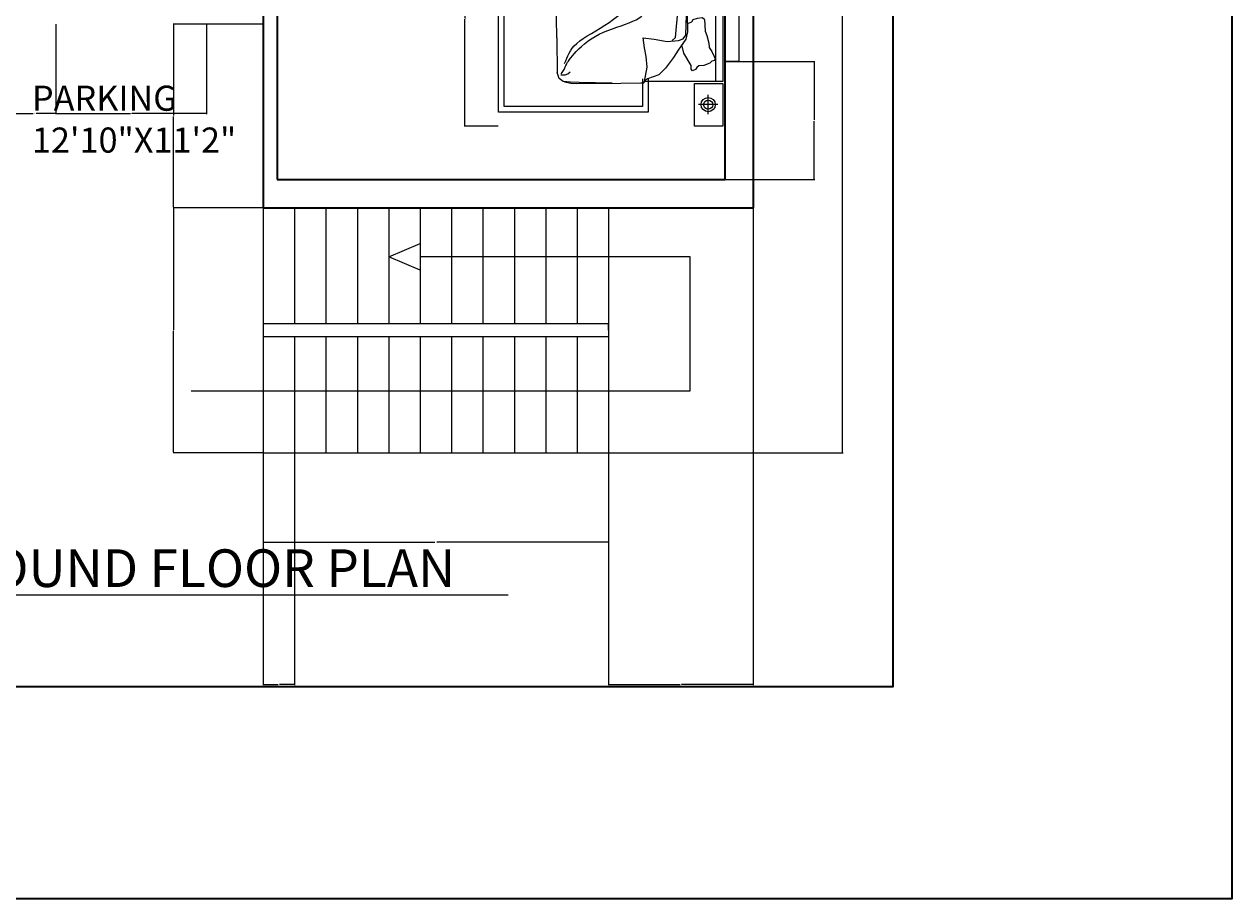
# Model space of a CAD drawing. Units: inches. Extents: x 1976 to 2558, y -977 to 2909.
# Tile 3 of 8: x 2173 to 2558, y 1748 to 2026. Entities that reach past the tile are written whole.
import ezdxf

# ---------------------------------------------------------------- set-up
doc = ezdxf.new("R2010")
doc.units = ezdxf.units.IN
for name, color, linetype, lineweight in [('A-ANNO-DIMS', 2, 'Continuous', 18), ('A-ANNO-SYMB', 2, 'Continuous', 18), ('A-ANNO-TEXT', 7, 'Continuous', 25), ('A-ANNO-TTLB', 7, 'Continuous', 35), ('A-AREA-IDEN', 7, 'Continuous', 18), ('A-FLOR-STRS', 7, 'Continuous', 25), ('A-FURN', 8, 'Continuous', 13), ('A-GLAZ', 4, 'Continuous', 18), ('A-WALL', 7, 'Continuous', 35)]:
    doc.layers.add(name, color=color, linetype=linetype, lineweight=lineweight)
doc.styles.get("Standard").update_dxf_attribs({"font": 'arial.ttf'})
doc.dimstyles.get("Standard").update_dxf_attribs({"dimtxt": 0.18, "dimasz": 0.18, "dimexe": 0.18, "dimexo": 0.0625, "dimgap": 0.09, "dimtad": 0, "dimtih": 1, "dimtoh": 1, "dimdec": 4, "dimzin": 0, "dimdsep": 46, "dimtxsty": 'Standard', "dimcen": 0.09, "dimadec": 0, "dimazin": 0, "dimtfac": 1, "dimtdec": 4, "dimtofl": 0, "dimtmove": 0, "dimatfit": 3, "dimfxl": 1, "dimtolj": 1, "dimtzin": 0, "dimarcsym": 0})

# ---------------------------------------------------------------- blocks, each defined once
blk = doc.blocks.new('BED-DOUBLE')
for p, q in [((69.87, 61.62), (63.73, 61.62)), ((66.8, 64.69), (66.8, 58.55)), ((20.15, 54.74), (18.94, 53.75)), ((22.42, 54.99), (20.15, 54.74)), ((25.18, 55.14), (22.42, 54.99)), ((35.73, 55.56), (25.18, 55.14)), ((55.41, 55.48), (35.73, 55.56)), ((56.88, 55.5), (55.41, 55.48)), ((57.51, 55.44), (56.88, 55.5)), ((58.41, 54.87), (71.47, 54.87)), ((18.94, 53.75), (18.3, 51.82)), ((18.55, 28.1), (18.3, 51.82)), ((66.5, 51.13), (67.81, 51.48)), ((60.75, 39.09), (59.91, 42.39)), ((68.04, 39.26), (68.74, 42.58)), ((68.74, 42.58), (68.6, 43.82)), ((60.42, 38.05), (60.75, 39.09)), ((68.42, 38.23), (68.04, 39.26)), ((60.63, 37.41), (60.42, 38.05)), ((61.72, 37.48), (60.63, 37.41)), ((62.3, 37.93), (61.72, 37.48)), ((63.04, 38.19), (62.3, 37.93)), ((64.58, 37.82), (63.04, 38.19)), ((66.65, 37.8), (64.58, 37.82)), ((67.64, 38.21), (66.65, 37.8)), ((68.39, 38.13), (67.64, 38.21)), ((68.39, 38.13), (67.64, 38.21)), ((68.39, 38.13), (68.42, 38.23)), ((65.64, 33.99), (65.86, 30.18)), ((18.55, 28.1), (18.55, 23.26)), ((65.86, 30.18), (66.35, 28.89)), ((66.35, 28.89), (67.01, 26.44)), ((18.55, 23.26), (18.68, 21.54)), ((61.33, 19.24), (59.08, 23.24)), ((67.01, 26.44), (67.13, 25.01)), ((67.13, 25.01), (67.97, 23.75)), ((67.13, 25.01), (67.97, 23.75)), ((67.97, 23.75), (68.81, 21.95)), ((18.68, 21.54), (18.68, 17.02)), ((61.37, 18.14), (61.33, 19.24)), ((65.36, 19.33), (63.79, 19.16)), ((67.32, 20.02), (65.36, 19.33)), ((68.1, 20.74), (67.32, 20.02)), ((19.39, 15.11), (18.68, 17.02)), ((19.85, 16.29), (21.2, 16.35)), ((21.2, 16.35), (22.12, 16.65)), ((22.12, 16.65), (22.82, 17.31)), ((61.78, 17.61), (61.37, 18.14)), ((62.78, 18.04), (61.78, 17.61)), ((63.18, 18.67), (62.78, 18.04)), ((63.79, 19.16), (63.18, 18.67)), ((20.62, 14.15), (19.39, 15.11)), ((22.9, 13.97), (20.62, 14.15)), ((21.04, 14.04), (23.05, 13.66)), ((25.67, 13.91), (22.9, 13.97)), ((23.05, 13.66), (24.99, 13.54)), ((24.99, 13.54), (38.97, 13.68)), ((36.23, 13.64), (25.67, 13.91)), ((38.97, 13.68), (45.35, 13.75)), ((46.53, 14.29), (46.57, 14.2)), ((66.8, 3.77), (66.8, 9.91)), ((69.87, 6.84), (63.73, 6.84))]:
    blk.add_line(p, q)
for points in [[(62.44, 68.46), (62.44, 54.92), (71.47, 54.92), (71.47, 68.46)], [(62.44, 0), (62.44, 13.54), (71.47, 13.54), (71.47, 0)]]:
    blk.add_lwpolyline(points, close=True)
for points in [[(47.73, 15.09), (47.73, 4.46), (0, 4.46), (0, 62.42), (47.73, 62.42), (47.73, 55.51)], [(45.92, 15.09), (45.92, 6.27), (1.81, 6.27), (1.81, 60.61), (45.92, 60.61), (45.92, 55.51)], [(46.51, 14.22), (47.31, 18.77), (47.06, 22.14), (46.5, 24.88), (46.05, 28.14), (49.6, 27.7), (53.74, 26.97), (57.39, 27.29), (58.87, 27.77), (59.72, 28.96), (59.98, 38.59), (59.57, 52.44), (58.73, 53.86), (57.9, 54.46), (57.82, 54.53)], [(58.65, 54.52), (59.13, 53.97), (59.77, 52.45), (60.21, 29.99), (59.63, 27.73), (57.24, 24.13), (55.74, 21.86), (53.24, 18.45), (51.03, 16.28), (47.47, 15), (46.54, 14.37)], [(71.47, 54.87), (71.47, 14.22), (46.61, 14.22)], [(55.37, 27.24), (56.41, 28.26), (57.19, 37.43), (57.04, 40.1), (56.37, 53.37), (55.53, 54.49), (54.4, 55.34)], [(57.55, 55.42), (57.97, 55.29), (58.3, 55.1), (58.41, 54.87), (58.64, 54.6), (58.65, 54.56)], [(69.21, 14.22), (69.21, 54.87)], [(59.99, 43.62), (60.51, 48.57), (60.69, 50), (60.38, 50.84), (60.47, 51.53), (61.01, 51.34), (61.95, 51.45), (64.12, 51.49), (66.5, 51.18)], [(68.6, 43.82), (67.86, 48.73), (67.62, 50.16), (67.9, 51.01), (67.81, 51.48)], [(21.07, 19.9), (21.44, 20.76), (21.79, 21.6), (22.14, 22.42), (22.52, 23.22), (22.95, 24.01), (23.48, 24.78), (24.13, 25.56), (24.93, 26.33), (25.9, 27.1), (27.01, 27.89), (28.25, 28.69), (29.59, 29.5), (30.98, 30.34), (32.41, 31.2), (33.84, 32.1), (35.25, 33.03), (36.61, 34), (37.91, 35), (39.14, 36), (40.28, 37), (41.34, 37.97), (42.3, 38.91), (43.16, 39.79), (43.9, 40.61), (44.52, 41.34), (44.99, 41.98), (45.3, 42.54), (45.43, 43.02), (45.35, 43.42), (45.05, 43.74), (44.51, 43.98), (43.7, 44.14)], [(20, 16.69), (20.29, 17.07), (20.52, 17.41), (20.72, 17.72), (20.88, 18.01), (21.02, 18.28), (21.14, 18.55), (21.26, 18.81), (21.37, 19.07), (21.5, 19.34), (21.64, 19.63), (21.82, 19.96), (22.04, 20.32), (22.31, 20.72), (22.64, 21.19), (23.05, 21.72), (23.54, 22.32), (24.12, 23.01), (24.8, 23.76), (25.57, 24.56), (26.43, 25.38), (27.39, 26.22), (28.43, 27.04), (29.56, 27.83), (30.78, 28.58), (32.09, 29.26), (33.45, 29.88), (34.86, 30.45), (36.28, 30.99), (37.7, 31.49), (39.08, 31.98), (40.41, 32.45), (41.66, 32.92), (42.81, 33.4), (43.84, 33.89), (44.73, 34.4), (45.46, 34.92), (46.02, 35.46), (46.39, 36.02), (46.55, 36.61), (46.48, 37.23)], [(65.64, 33.99), (64.89, 34.52), (63.32, 34.27), (61.94, 33.89), (61.5, 33.14), (60.37, 32.7), (60.16, 32.7)], [(59.08, 23.24), (58.42, 25.91)], [(68.1, 20.74), (68.93, 20.99), (69.11, 21.53), (68.81, 21.95)], [(45.41, 13.75), (46.29, 13.81), (46.55, 14.07), (46.61, 14.22)]]:
    blk.add_lwpolyline(points)
for centre, radius in [((66.8, 61.62), 2.26), ((66.8, 61.62), 1.45), ((66.8, 6.84), 2.26), ((66.8, 6.84), 1.45)]:
    blk.add_circle(centre, radius)
blk = doc.blocks.new('WIN-60-PLAN')
for p, q in [((4.5, 60), (0, 60)), ((0, 60), (9, 60)), ((4.5, 0), (4.5, 60)), ((0, 0), (9, 0)), ((9, 0), (4.5, 0))]:
    blk.add_line(p, q)
blk = doc.blocks.new('*D16')
at = {"layer": 'A-ANNO-DIMS', "color": 0, "lineweight": -2, "transparency": 16777216}
for p, q in [((2324.3, 2062.48), (2313.46, 2062.48)), ((2313.64, 2062.3), (2313.64, 2028.43)), ((2313.64, 1994.19), (2313.64, 2028.06)), ((2324.3, 1994.01), (2313.46, 1994.01))]:
    blk.add_line(p, q, dxfattribs=at)
at = {"layer": 'A-ANNO-DIMS', "color": 0, "transparency": 16777216}
for points in [[(2313.61, 2062.3), (2313.67, 2062.3), (2313.64, 2062.48)], [(2313.61, 1994.19), (2313.67, 1994.19), (2313.64, 1994.01)]]:
    blk.add_solid(points, dxfattribs=at)
at = {"layer": 'Defpoints', "color": 0, "transparency": 16777216}
for p in [(2313.64, 2062.48), (2324.36, 2062.48), (2324.36, 1994.01)]:
    blk.add_point(p, dxfattribs=at)
at = {"layer": 'A-ANNO-DIMS', "color": 0, "transparency": 16777216, "insert": (2313.64, 2028.25), "char_height": 0.18, "attachment_point": 5}
blk.add_mtext('\\A1;68 TYP.', dxfattribs=at)
blk = doc.blocks.new('*D24')
at = {"layer": 'A-ANNO-DIMS', "color": 0, "lineweight": -2, "transparency": 16777216}
for p, q in [((2405.5, 2383.48), (2434.12, 2383.48)), ((2433.94, 2383.3), (2433.94, 2136.91)), ((2433.94, 1890.16), (2433.94, 2136.55)), ((2359.5, 1889.98), (2434.12, 1889.98))]:
    blk.add_line(p, q, dxfattribs=at)
at = {"layer": 'A-ANNO-DIMS', "color": 0, "transparency": 16777216}
for points in [[(2433.91, 2383.3), (2433.97, 2383.3), (2433.94, 2383.48)], [(2433.91, 1890.16), (2433.97, 1890.16), (2433.94, 1889.98)]]:
    blk.add_solid(points, dxfattribs=at)
at = {"layer": 'Defpoints', "color": 0, "transparency": 16777216}
for p in [(2405.44, 2383.48), (2433.94, 2383.48), (2359.44, 1889.98)]:
    blk.add_point(p, dxfattribs=at)
at = {"layer": 'A-ANNO-DIMS', "color": 0, "transparency": 16777216, "insert": (2433.94, 2136.73), "char_height": 0.18, "attachment_point": 5}
blk.add_mtext('\\A1;493.5', dxfattribs=at)
blk = doc.blocks.new('*D25')
at = {"layer": 'A-ANNO-DIMS', "color": 0, "lineweight": -2, "transparency": 16777216}
for p, q in [((2249.38, 1967.98), (2220.76, 1967.98)), ((2220.94, 1967.8), (2220.94, 1929.16)), ((2220.94, 1890.16), (2220.94, 1928.8)), ((2249.38, 1889.98), (2220.76, 1889.98))]:
    blk.add_line(p, q, dxfattribs=at)
at = {"layer": 'A-ANNO-DIMS', "color": 0, "transparency": 16777216}
for points in [[(2220.91, 1967.8), (2220.97, 1967.8), (2220.94, 1967.98)], [(2220.91, 1890.16), (2220.97, 1890.16), (2220.94, 1889.98)]]:
    blk.add_solid(points, dxfattribs=at)
at = {"layer": 'Defpoints', "color": 0, "transparency": 16777216}
for p in [(2220.94, 1967.98), (2249.44, 1967.98), (2249.44, 1889.98)]:
    blk.add_point(p, dxfattribs=at)
at = {"layer": 'A-ANNO-DIMS', "color": 0, "transparency": 16777216, "insert": (2220.94, 1928.98), "char_height": 0.18, "attachment_point": 5}
blk.add_mtext('\\A1;78', dxfattribs=at)
blk = doc.blocks.new('*D26')
at = {"layer": 'A-ANNO-DIMS', "color": 0, "lineweight": -2, "transparency": 16777216}
for p, q in [((2249.44, 1889.92), (2249.44, 1861.3)), ((2359.44, 1889.92), (2359.44, 1861.3)), ((2249.62, 1861.48), (2304.16, 1861.48)), ((2359.26, 1861.48), (2304.72, 1861.48))]:
    blk.add_line(p, q, dxfattribs=at)
at = {"layer": 'A-ANNO-DIMS', "color": 0, "transparency": 16777216}
for points in [[(2249.62, 1861.51), (2249.62, 1861.45), (2249.44, 1861.48)], [(2359.26, 1861.51), (2359.26, 1861.45), (2359.44, 1861.48)]]:
    blk.add_solid(points, dxfattribs=at)
at = {"layer": 'Defpoints', "color": 0, "transparency": 16777216}
for p in [(2249.44, 1889.98), (2359.44, 1889.98), (2249.44, 1861.48)]:
    blk.add_point(p, dxfattribs=at)
at = {"layer": 'A-ANNO-DIMS', "color": 0, "transparency": 16777216, "insert": (2304.44, 1861.48), "char_height": 0.18, "attachment_point": 5}
blk.add_mtext('\\A1;110', dxfattribs=at)
blk = doc.blocks.new('*D27')
at = {"layer": 'A-ANNO-DIMS', "color": 0, "lineweight": -2, "transparency": 16777216}
for p, q in [((2405.44, 1967.92), (2405.44, 1815.97)), ((2359.44, 1889.92), (2359.44, 1815.97)), ((2359.62, 1816.15), (2382.22, 1816.15)), ((2405.26, 1816.15), (2382.66, 1816.15))]:
    blk.add_line(p, q, dxfattribs=at)
at = {"layer": 'A-ANNO-DIMS', "color": 0, "transparency": 16777216}
for points in [[(2359.62, 1816.18), (2359.62, 1816.12), (2359.44, 1816.15)], [(2405.26, 1816.18), (2405.26, 1816.12), (2405.44, 1816.15)]]:
    blk.add_solid(points, dxfattribs=at)
at = {"layer": 'Defpoints', "color": 0, "transparency": 16777216}
for p in [(2405.44, 1967.98), (2359.44, 1889.98), (2405.44, 1816.15)]:
    blk.add_point(p, dxfattribs=at)
at = {"layer": 'A-ANNO-DIMS', "color": 0, "transparency": 16777216, "insert": (2382.44, 1816.15), "char_height": 0.18, "attachment_point": 5}
blk.add_mtext('\\A1;46', dxfattribs=at)
blk = doc.blocks.new('*D37')
at = {"layer": 'A-ANNO-DIMS', "color": 0, "lineweight": -2, "transparency": 16777216}
for p, q in [((2396.5, 2014.62), (2425.12, 2014.62)), ((2424.94, 2014.44), (2424.94, 1995.98)), ((2424.94, 1977.16), (2424.94, 1995.62)), ((2396.5, 1976.98), (2425.12, 1976.98))]:
    blk.add_line(p, q, dxfattribs=at)
at = {"layer": 'A-ANNO-DIMS', "color": 0, "transparency": 16777216}
for points in [[(2424.91, 2014.44), (2424.97, 2014.44), (2424.94, 2014.62)], [(2424.91, 1977.16), (2424.97, 1977.16), (2424.94, 1976.98)]]:
    blk.add_solid(points, dxfattribs=at)
at = {"layer": 'Defpoints', "color": 0, "transparency": 16777216}
for p in [(2396.44, 2014.62), (2396.44, 1976.98), (2424.94, 1976.98)]:
    blk.add_point(p, dxfattribs=at)
at = {"layer": 'A-ANNO-DIMS', "color": 0, "transparency": 16777216, "insert": (2424.94, 1995.8), "char_height": 0.18, "attachment_point": 5}
blk.add_mtext('\\A1;37.64', dxfattribs=at)
blk = doc.blocks.new('*D41')
at = {"layer": 'A-ANNO-DIMS', "color": 0, "lineweight": -2, "transparency": 16777216}
for p, q in [((2249.38, 2026.48), (2220.76, 2026.48)), ((2220.94, 2026.3), (2220.94, 1997.41)), ((2220.94, 1968.16), (2220.94, 1997.05)), ((2249.38, 1967.98), (2220.76, 1967.98))]:
    blk.add_line(p, q, dxfattribs=at)
at = {"layer": 'A-ANNO-DIMS', "color": 0, "transparency": 16777216}
for points in [[(2220.91, 2026.3), (2220.97, 2026.3), (2220.94, 2026.48)], [(2220.91, 1968.16), (2220.97, 1968.16), (2220.94, 1967.98)]]:
    blk.add_solid(points, dxfattribs=at)
at = {"layer": 'Defpoints', "color": 0, "transparency": 16777216}
for p in [(2220.94, 2026.48), (2249.44, 2026.48), (2249.44, 1967.98)]:
    blk.add_point(p, dxfattribs=at)
at = {"layer": 'A-ANNO-DIMS', "color": 0, "transparency": 16777216, "insert": (2220.94, 1997.23), "char_height": 0.18, "attachment_point": 5}
blk.add_mtext('\\A1;58.5', dxfattribs=at)
blk = doc.blocks.new('*D44')
at = {"layer": 'A-ANNO-DIMS', "color": 0, "lineweight": -2, "transparency": 16777216}
for p, q in [((2169.89, 2026.42), (2169.89, 1997.8)), ((2183.44, 2026.42), (2183.44, 1997.8)), ((2170.07, 1997.98), (2176.21, 1997.98)), ((2183.26, 1997.98), (2177.12, 1997.98))]:
    blk.add_line(p, q, dxfattribs=at)
at = {"layer": 'A-ANNO-DIMS', "color": 0, "transparency": 16777216}
for points in [[(2170.07, 1998.01), (2170.07, 1997.95), (2169.89, 1997.98)], [(2183.26, 1998.01), (2183.26, 1997.95), (2183.44, 1997.98)]]:
    blk.add_solid(points, dxfattribs=at)
at = {"layer": 'Defpoints', "color": 0, "transparency": 16777216}
for p in [(2169.89, 2026.48), (2183.44, 2026.48), (2169.89, 1997.98)]:
    blk.add_point(p, dxfattribs=at)
at = {"layer": 'A-ANNO-DIMS', "color": 0, "transparency": 16777216, "insert": (2176.66, 1997.98), "char_height": 0.18, "attachment_point": 5}
blk.add_mtext('\\A1;13.552', dxfattribs=at)
blk = doc.blocks.new('*D45')
at = {"layer": 'A-ANNO-DIMS', "color": 0, "lineweight": -2, "transparency": 16777216}
for p, q in [((2183.44, 2026.42), (2183.44, 1997.8)), ((2231.44, 2026.42), (2231.44, 1997.8)), ((2183.62, 1997.98), (2207.22, 1997.98)), ((2231.26, 1997.98), (2207.66, 1997.98))]:
    blk.add_line(p, q, dxfattribs=at)
at = {"layer": 'A-ANNO-DIMS', "color": 0, "transparency": 16777216}
for points in [[(2183.62, 1998.01), (2183.62, 1997.95), (2183.44, 1997.98)], [(2231.26, 1998.01), (2231.26, 1997.95), (2231.44, 1997.98)]]:
    blk.add_solid(points, dxfattribs=at)
at = {"layer": 'Defpoints', "color": 0, "transparency": 16777216}
for p in [(2183.44, 2026.48), (2231.44, 2026.48), (2183.44, 1997.98)]:
    blk.add_point(p, dxfattribs=at)
at = {"layer": 'A-ANNO-DIMS', "color": 0, "transparency": 16777216, "insert": (2207.44, 1997.98), "char_height": 0.18, "attachment_point": 5}
blk.add_mtext('\\A1;48', dxfattribs=at)
blk = doc.blocks.new('*D46')
at = {"layer": 'A-ANNO-DIMS', "color": 0, "lineweight": -2, "transparency": 16777216}
for p, q in [((2249.44, 1889.92), (2249.44, 1815.97)), ((2259.44, 1889.92), (2259.44, 1815.97)), ((2249.62, 1816.15), (2254.23, 1816.15)), ((2259.26, 1816.15), (2254.65, 1816.15))]:
    blk.add_line(p, q, dxfattribs=at)
at = {"layer": 'A-ANNO-DIMS', "color": 0, "transparency": 16777216}
for points in [[(2249.62, 1816.18), (2249.62, 1816.12), (2249.44, 1816.15)], [(2259.26, 1816.18), (2259.26, 1816.12), (2259.44, 1816.15)]]:
    blk.add_solid(points, dxfattribs=at)
at = {"layer": 'Defpoints', "color": 0, "transparency": 16777216}
for p in [(2249.44, 1889.98), (2259.44, 1889.98), (2259.44, 1816.15)]:
    blk.add_point(p, dxfattribs=at)
at = {"layer": 'A-ANNO-DIMS', "color": 0, "transparency": 16777216, "insert": (2254.44, 1816.15), "char_height": 0.18, "attachment_point": 5}
blk.add_mtext('\\A1;10', dxfattribs=at)

msp = doc.modelspace()

# ---------------------------------------------------------------- linework, layer by layer
at = {"layer": 'A-ANNO-SYMB'}
for p, q in [((2289.4385, 1952.4004), (2299.4385, 1956.6538)), ((2299.4385, 1956.6538), (2299.4385, 1948.1487)), ((2299.4385, 1948.1487), (2289.4385, 1952.4004)), ((2385.3927, 1952.4004), (2299.4385, 1952.4004)), ((2385.3927, 1909.6881), (2385.3927, 1952.4004)), ((2226.5284, 1909.6881), (2385.3927, 1909.6881))]:
    msp.add_line(p, q, dxfattribs=at)
at = {"layer": 'A-ANNO-TEXT'}
msp.add_line((2140.9443, 1844.6463), (2327.4413, 1844.6463), dxfattribs=at)
at = {"layer": 'A-ANNO-TTLB'}
for points in [[(1975.8545, 2909.3429), (2557.9168, 2909.3429), (2557.9168, 1747.8598), (1975.8545, 1747.8598)], [(2055.4343, 2428.9091), (2450.0007, 2428.9091), (2450.0007, 1815.3916), (2055.4343, 1815.3916)]]:
    msp.add_lwpolyline(points, close=True, dxfattribs=at)
at = {"layer": 'A-FLOR-STRS'}
for p, q in [((2249.4385, 1967.9789), (2249.4385, 1889.9789)), ((2259.4385, 1967.9789), (2259.4385, 1930.9789)), ((2269.4385, 1967.9789), (2269.4385, 1930.9789)), ((2279.4385, 1967.9789), (2279.4385, 1930.9789)), ((2289.4385, 1967.9789), (2289.4385, 1930.9789)), ((2299.4385, 1967.9789), (2299.4385, 1930.9789)), ((2309.4385, 1967.9789), (2309.4385, 1930.9789)), ((2319.4385, 1967.9789), (2319.4385, 1930.9789)), ((2329.4385, 1967.9789), (2329.4385, 1930.9789)), ((2339.4385, 1967.9789), (2339.4385, 1930.9789)), ((2349.4385, 1967.9789), (2349.4385, 1930.9789)), ((2359.4385, 1967.9789), (2359.4385, 1889.9789)), ((2359.4385, 1930.9789), (2249.4385, 1930.9789)), ((2249.4385, 1930.9789), (2249.4385, 1928.9789)), ((2359.4385, 1928.9789), (2359.4385, 1930.9789)), ((2249.4385, 1928.9789), (2249.4385, 1926.9789)), ((2249.4385, 1926.9789), (2359.4385, 1926.9789)), ((2259.4385, 1926.9789), (2259.4385, 1889.9789)), ((2269.4385, 1926.9789), (2269.4385, 1889.9789)), ((2279.4385, 1926.9789), (2279.4385, 1889.9789)), ((2289.4385, 1926.9789), (2289.4385, 1889.9789)), ((2299.4385, 1926.9789), (2299.4385, 1889.9789)), ((2309.4385, 1926.9789), (2309.4385, 1889.9789)), ((2319.4385, 1926.9789), (2319.4385, 1889.9789)), ((2329.4385, 1926.9789), (2329.4385, 1889.9789)), ((2339.4385, 1926.9789), (2339.4385, 1889.9789)), ((2349.4385, 1926.9789), (2349.4385, 1889.9789)), ((2359.4385, 1928.9789), (2359.4385, 1928.9789)), ((2249.4385, 1889.9789), (2359.4385, 1889.9789))]:
    msp.add_line(p, q, dxfattribs=at)
at = {"layer": 'A-WALL'}
for p, q in [((2405.4385, 2383.4789), (2405.4385, 1967.9789)), ((2249.4385, 2113.4789), (2249.4385, 1967.9789)), ((2253.9385, 2108.9789), (2253.9385, 1976.9789)), ((2396.4385, 2108.9789), (2396.4385, 1976.9789)), ((2253.9385, 1976.9789), (2396.4385, 1976.9789)), ((2249.4385, 1967.9789), (2405.4385, 1967.9789))]:
    msp.add_line(p, q, dxfattribs=at)

# ---------------------------------------------------------------- block references
at = {"layer": 'A-FURN'}
msp.add_blockref('BED-DOUBLE', (2324.364, 1994.015), dxfattribs=at)
at = {"layer": 'A-GLAZ', "extrusion": (0, 0, -1), "zscale": -1, "rotation": 180}
msp.add_blockref('WIN-60-PLAN', (-2396.438, 2074.6199), dxfattribs=at)

# ---------------------------------------------------------------- texts
at = {"layer": 'A-ANNO-TEXT', "insert": (2140.8831, 1859.1948), "char_height": 12, "attachment_point": 1}
msp.add_mtext_dynamic_manual_height_columns('GROUND FLOOR PLAN', width=194.661531, gutter_width=12.5, heights=[0], dxfattribs=at)
at = {"layer": 'A-AREA-IDEN', "insert": (2175.812, 2006.8868), "char_height": 8, "attachment_point": 1}
msp.add_mtext_dynamic_manual_height_columns('PARKING\\P12\'10"X11\'2"', width=183.810377, gutter_width=12.5, heights=[0], dxfattribs=at)

# ---------------------------------------------------------------- dimensions: what is measured, and where the dimension line sits
at = {"layer": 'A-ANNO-DIMS'}
for base, p1, p2, angle, override, picture, middle in [((2433.9385, 2383.4789), (2359.4385, 1889.9789), (2405.4385, 2383.4789), 90, {"dimdec": 1, "dimlfac": 1, "dimrnd": 0, "dimzin": 0, "dimdsep": 46, "dimlunit": 2}, '*D24', (2433.9385, 2136.7289)), ((2169.8866, 1997.9789), (2183.4385, 2026.4789), (2169.8866, 2026.4789), 180, {"dimdec": 3, "dimlfac": 1, "dimrnd": 0, "dimzin": 0, "dimdsep": 46, "dimlunit": 2}, '*D44', (2176.6625, 1997.9789)), ((2183.4385, 1997.9789), (2231.4385, 2026.4789), (2183.4385, 2026.4789), 180, {"dimdec": 0, "dimlfac": 1, "dimrnd": 0, "dimzin": 0, "dimdsep": 46, "dimlunit": 2}, '*D45', (2207.4385, 1997.9789)), ((2220.9385, 2026.4789), (2249.4385, 1967.9789), (2249.4385, 2026.4789), 90, {"dimdec": 1, "dimlfac": 1, "dimrnd": 0, "dimzin": 0, "dimdsep": 46, "dimlunit": 2}, '*D41', (2220.9385, 1997.2289)), ((2424.9385, 1976.9789), (2396.4385, 2014.62), (2396.4385, 1976.9789), 270, {"dimdec": 2, "dimlfac": 1, "dimrnd": 0, "dimzin": 0, "dimdsep": 46, "dimlunit": 2}, '*D37', (2424.9385, 1995.7994)), ((2220.9385, 1967.9789), (2249.4385, 1889.9789), (2249.4385, 1967.9789), 90, {"dimdec": 0, "dimlfac": 1, "dimrnd": 0, "dimzin": 0, "dimdsep": 46, "dimlunit": 2}, '*D25', (2220.9385, 1928.9789)), ((2249.4385, 1861.4789), (2359.4385, 1889.9789), (2249.4385, 1889.9789), 180, {"dimdec": 0, "dimlfac": 1, "dimrnd": 0, "dimzin": 0, "dimdsep": 46, "dimlunit": 2}, '*D26', (2304.4385, 1861.4789))]:
    dim = msp.add_linear_dim(base=base, p1=p1, p2=p2, angle=angle, dimstyle='Standard', override=override, dxfattribs=at)
    dim.commit()
    dim.dimension.update_dxf_attribs({"geometry": picture, "text_midpoint": middle})
dim = msp.add_linear_dim(base=(2313.6434, 2062.4772), p1=(2324.3642, 1994.0146), p2=(2324.3642, 2062.4772), angle=90, text='<> TYP.', dimstyle='Standard', override={"dimdec": 0, "dimlfac": 1, "dimrnd": 0, "dimzin": 0, "dimdsep": 46, "dimlunit": 2}, dxfattribs=at)
dim.commit()
dim.dimension.update_dxf_attribs({"geometry": '*D16', "text_midpoint": (2313.6434, 2028.2459)})
for base, p1, p2, picture, middle in [((2405.4385, 1816.1463), (2359.4385, 1889.9789), (2405.4385, 1967.9789), '*D27', (2382.4385, 1816.1463)), ((2259.4385, 1816.1463), (2249.4385, 1889.9789), (2259.4385, 1889.9789), '*D46', (2254.4385, 1816.1463))]:
    dim = msp.add_linear_dim(base=base, p1=p1, p2=p2, dimstyle='Standard', override={"dimdec": 0, "dimlfac": 1, "dimrnd": 0, "dimzin": 0, "dimdsep": 46, "dimlunit": 2}, dxfattribs=at)
    dim.commit()
    dim.dimension.update_dxf_attribs({"geometry": picture, "text_midpoint": middle})

doc.saveas('drawing.dxf')
